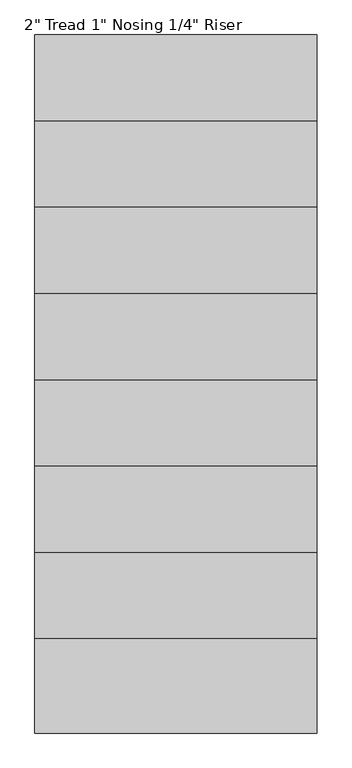
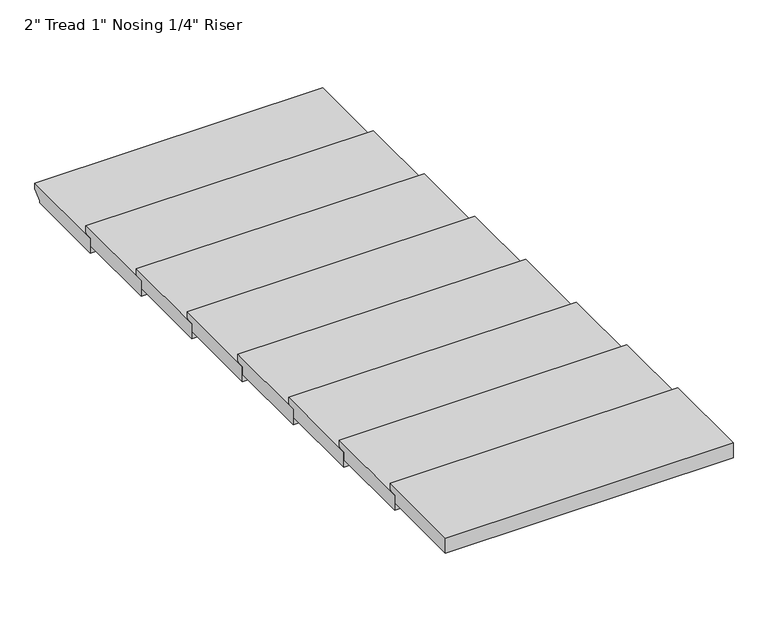
"""IFC4 building model written with IfcOpenShell, lengths in millimetres: stair flight geometry."""

from ifc_helpers import new_model, si_unit, frame, origin, place, context, project, spatial, polyline, outline, extrude, source, transform, mapped, element, save


def stair_flight_cd86263c(model_context):
    return source(origin(), model_context, "Body", "SweptSolid", [
        extrude(outline(polyline([(12995.2419954, 3454.4), (13300.0419954, 3454.4), (13300.0419954, 3435.35), (13274.6419954, 3409.95), (13274.6419954, 3403.6), (12995.2419954, 3403.6), (12995.2419954, 3454.4)])), frame((-5762.1737939, 0.0, 0.0), z_axis=(1.0, 0.0, 0.0), x_axis=(0.0, 1.0, 0.0)), (0.0, 0.0, 1.0), 914.4),
        extrude(outline(polyline([(12715.8419954, 3479.8), (13020.6419954, 3479.8), (13020.6419954, 3460.75), (12995.2419954, 3435.35), (12995.2419954, 3429.0), (12715.8419954, 3429.0), (12715.8419954, 3479.8)])), frame((-5762.1737939, 0.0, 0.0), z_axis=(1.0, 0.0, 0.0), x_axis=(0.0, 1.0, 0.0)), (0.0, 0.0, 1.0), 914.4),
        extrude(outline(polyline([(12436.4419954, 3505.2), (12741.2419954, 3505.2), (12741.2419954, 3486.15), (12715.8419954, 3460.75), (12715.8419954, 3454.4), (12436.4419954, 3454.4), (12436.4419954, 3505.2)])), frame((-5762.1737939, 0.0, 0.0), z_axis=(1.0, 0.0, 0.0), x_axis=(0.0, 1.0, 0.0)), (0.0, 0.0, 1.0), 914.4),
        extrude(outline(polyline([(12157.0419954, 3530.6), (12461.8419954, 3530.6), (12461.8419954, 3511.55), (12436.4419954, 3486.15), (12436.4419954, 3479.8), (12157.0419954, 3479.8), (12157.0419954, 3530.6)])), frame((-5762.1737939, 0.0, 0.0), z_axis=(1.0, 0.0, 0.0), x_axis=(0.0, 1.0, 0.0)), (0.0, 0.0, 1.0), 914.4),
        extrude(outline(polyline([(11877.6419954, 3556.0), (12182.4419954, 3556.0), (12182.4419954, 3536.95), (12157.0419954, 3511.55), (12157.0419954, 3505.2), (11877.6419954, 3505.2), (11877.6419954, 3556.0)])), frame((-5762.1737939, 0.0, 0.0), z_axis=(1.0, 0.0, 0.0), x_axis=(0.0, 1.0, 0.0)), (0.0, 0.0, 1.0), 914.4),
        extrude(outline(polyline([(11598.2419954, 3581.4), (11903.0419954, 3581.4), (11903.0419954, 3562.35), (11877.6419954, 3536.95), (11877.6419954, 3530.6), (11598.2419954, 3530.6), (11598.2419954, 3581.4)])), frame((-5762.1737939, 0.0, 0.0), z_axis=(1.0, 0.0, 0.0), x_axis=(0.0, 1.0, 0.0)), (0.0, 0.0, 1.0), 914.4),
        extrude(outline(polyline([(11318.8419954, 3606.8), (11623.6419954, 3606.8), (11623.6419954, 3587.75), (11598.2419954, 3562.35), (11598.2419954, 3556.0), (11318.8419954, 3556.0), (11318.8419954, 3606.8)])), frame((-5762.1737939, 0.0, 0.0), z_axis=(1.0, 0.0, 0.0), x_axis=(0.0, 1.0, 0.0)), (0.0, 0.0, 1.0), 914.4),
        extrude(outline(polyline([(11039.4419954, 3632.2), (11344.2419954, 3632.2), (11344.2419954, 3613.15), (11318.8419954, 3587.75), (11318.8419954, 3581.4), (11039.4419954, 3581.4), (11039.4419954, 3632.2)])), frame((-5762.1737939, 0.0, 0.0), z_axis=(1.0, 0.0, 0.0), x_axis=(0.0, 1.0, 0.0)), (0.0, 0.0, 1.0), 914.4),
    ])


if __name__ == "__main__":
    model = new_model("IFC4")
    model_context = context("Model", 3, world=origin())
    ifc_project = project(units=[si_unit("LENGTHUNIT", "METRE", prefix="MILLI")], contexts=[model_context])
    site = spatial("IfcSite", under=ifc_project)
    building = spatial("IfcBuilding", under=site)
    placement = place(None, origin())
    stair_flight_shape = stair_flight_cd86263c(model_context)
    element("IfcStairFlight", 1, ObjectType="2\" Tread 1\" Nosing 1/4\" Riser", at=placement, inside=building, context=model_context, shape_type="MappedRepresentation", body=[
        mapped(stair_flight_shape, transform((0.0, 0.0, 0.0), x_axis=(1.0, 0.0, 0.0), y_axis=(0.0, 1.0, 0.0), z_axis=(0.0, 0.0, 1.0))),
    ])
    save(model, "model.ifc")
